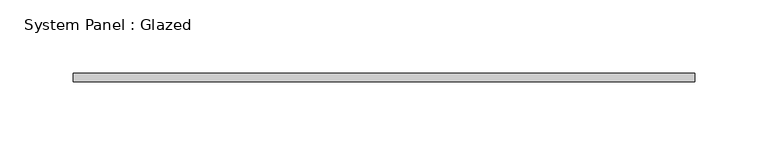
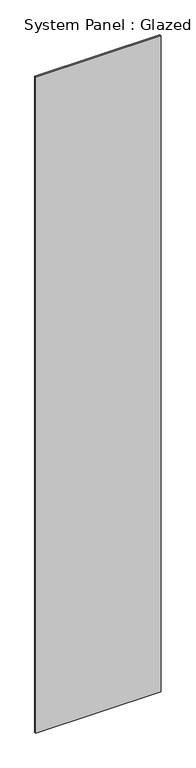
"""IFC4 building model written with IfcOpenShell, lengths in millimetres: plate geometry, System Panel : Glazed."""

from ifc_helpers import new_model, si_unit, origin, origin_with_axes, place, context, project, spatial, polyline, outline, extrude, source, transform, mapped, element, save


def system_panel_glazed_bc7b3e81(model_context):
    return source(origin(), model_context, "Body", "SweptSolid", [
        extrude(outline(polyline([(212.5, 34.0), (-212.5, 34.0), (-212.5, 40.0), (212.5, 40.0), (212.5, 34.0)])), origin_with_axes(), (0.0, 0.0, 1.0), 2350.0),
    ])


if __name__ == "__main__":
    model = new_model("IFC4")
    model_context = context("Model", 3, world=origin())
    ifc_project = project(units=[si_unit("LENGTHUNIT", "METRE", prefix="MILLI")], contexts=[model_context])
    site = spatial("IfcSite", under=ifc_project)
    building = spatial("IfcBuilding", under=site)
    placement = place(None, origin())
    system_panel_glazed_shape = system_panel_glazed_bc7b3e81(model_context)
    element("IfcPlate", 1, ObjectType="System Panel : Glazed", at=placement, inside=building, context=model_context, shape_type="MappedRepresentation", body=[
        mapped(system_panel_glazed_shape, transform((0.0, 0.0, 0.0), x_axis=(1.0, 0.0, 0.0), y_axis=(0.0, 1.0, 0.0), z_axis=(0.0, 0.0, 1.0))),
    ])
    save(model, "model.ifc")

# Revit data of these elements
# Type "System Panel : Glazed"
#   Construction Type Id = "GSP4R"
#   Analytic Construction = "1/8 in Pilkington single glazing"
#   Visual Light Transmittance = 0.9
#   Solar Heat Gain Coefficient = 0.86
#   Heat Transfer Coefficient (U) = 6.7069 W/(m²·K)
#   Define Thermal Properties by = 1
# Element 1 (IfcPlate, "System Panel : Glazed")
#   Materials on its faces: "Default New Material(6)"
# Materials
#   "Default New Material(6)": class "Generic", colour RGB 191 25 25, transparency 0.9, Cost = 0
